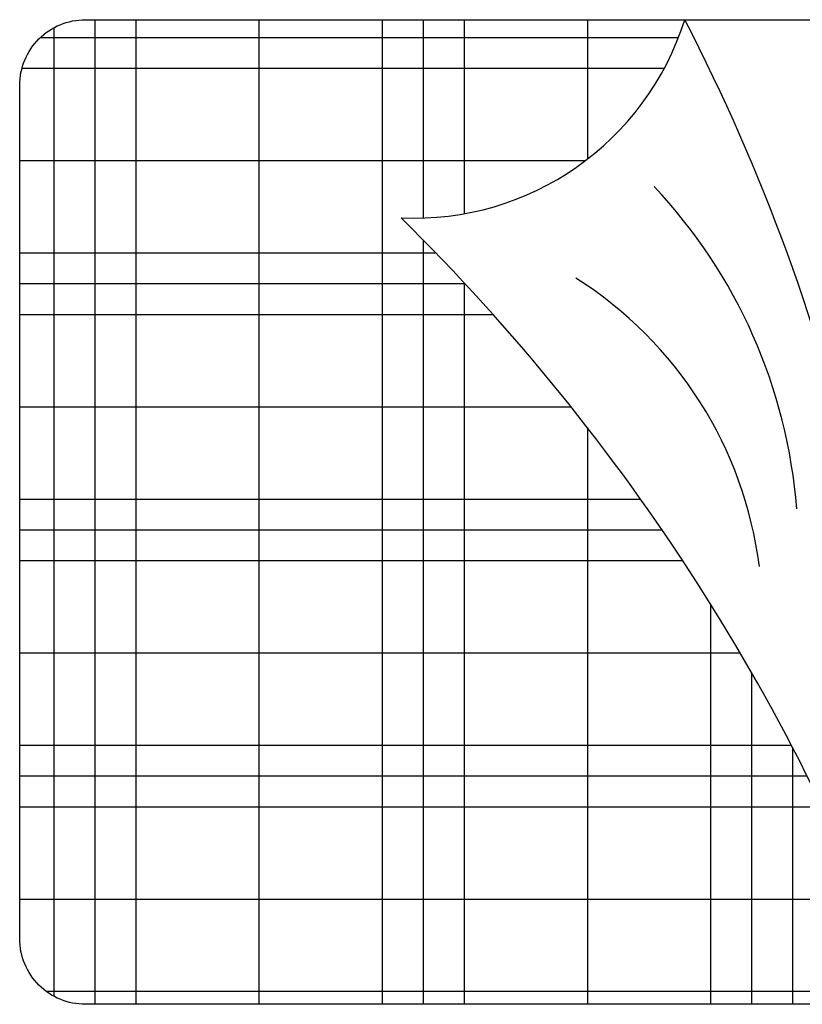
# Model space of a CAD drawing. Units: inches. Extents: x 3064 to 19385, y 846 to 15425.
# Tile 38 of 108: x 5255 to 5302, y 1030 to 1089. Entities that reach past the tile are written whole.
import ezdxf

# ---------------------------------------------------------------- set-up
doc = ezdxf.new("R2010")
doc.units = ezdxf.units.IN
doc.layers.add('A-FLOR-FIXT', color=9, linetype='Continuous', lineweight=18)
doc.layers.add('BLOCK', color=6, linetype='Continuous')

# ---------------------------------------------------------------- blocks, each defined once
blk = doc.blocks.new('*X5')
at = {"color": 0}
for p, q in [((276.598, 451.25), (280.51, 451.25)), ((275.455, 450.625), (280.51, 450.625)), ((274.411, 450), (280.51, 450)), ((265.51, 448.125), (267.634, 448.125)), ((271.723, 448.125), (280.51, 448.125)), ((265.51, 446.25), (268.465, 446.25)), ((269.519, 446.25), (280.51, 446.25)), ((265.51, 445.625), (268.531, 445.625)), ((268.866, 445.625), (280.51, 445.625)), ((265.51, 445), (280.51, 445)), ((265.51, 443.125), (280.51, 443.125)), ((265.51, 441.25), (280.51, 441.25)), ((265.51, 440.625), (280.51, 440.625)), ((265.634, 440), (280.386, 440))]:
    blk.add_line(p, q, dxfattribs=at)
blk = doc.blocks.new('*X6')
at = {"color": 0}
for p, q in [((280.312, 439.886), (280.312, 452.896)), ((278.906, 439.482), (278.906, 452.338)), ((277.5, 439.482), (277.5, 451.702)), ((277.031, 439.482), (277.031, 451.471)), ((276.562, 439.482), (276.562, 451.231)), ((275.156, 439.482), (275.156, 450.451)), ((273.75, 439.482), (273.75, 449.576)), ((265.781, 439.797), (265.781, 449.511)), ((266.25, 439.517), (266.25, 449.296)), ((273.281, 439.482), (273.281, 449.261)), ((272.812, 439.482), (272.812, 448.934)), ((267.656, 439.482), (267.656, 448.095)), ((271.406, 439.482), (271.406, 447.876)), ((270, 439.482), (270, 446.689)), ((269.531, 439.482), (269.531, 446.262)), ((269.062, 439.482), (269.062, 445.817))]:
    blk.add_line(p, q, dxfattribs=at)
blk = doc.blocks.new('A$C52E67D0D')
at = {"layer": 'BLOCK'}
blk.add_lwpolyline([(1901, 0), (601, 0, -0.414214), (501, 100), (501, 1700, -0.414214), (601, 1800), (1901, 1800, -0.414214), (2001, 1700), (2001, 100, -0.414214)], format="xyb", close=True, dxfattribs=at)
for centre, radius, start, end in [((1888.6, -1664.5), 3015.3, 87.8642, 117.4001), ((3101, -1685.8), 3227.7, 109.926, 135.3977), ((1308.8, 377.9), 807.6, 94.4436, 133.2788), ((1410.8, 520.2), 610.8, 97.2157, 147.6656), ((371.4, 600.4), 432, 357.3792, 72.5379)]:
    blk.add_arc(centre, radius, start, end, dxfattribs=at)
at = {"layer": 'BLOCK', "xscale": 100, "yscale": 100, "zscale": 100}
for name in ['*X6', '*X5']:
    blk.add_blockref(name, (-26050, -43948.2), dxfattribs=at)

msp = doc.modelspace()

# ---------------------------------------------------------------- block references
at = {"layer": 'A-FLOR-FIXT', "xscale": 0.039370099999992, "yscale": 0.039370099999992, "zscale": 0.039370099999992, "rotation": 270}
msp.add_blockref('A$C52E67D0D', (5255.151, 1108.348), dxfattribs=at)

doc.saveas('drawing.dxf')
